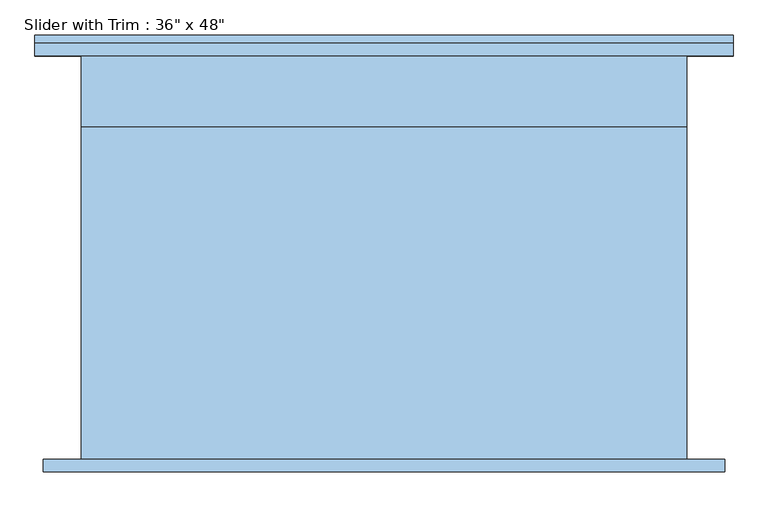
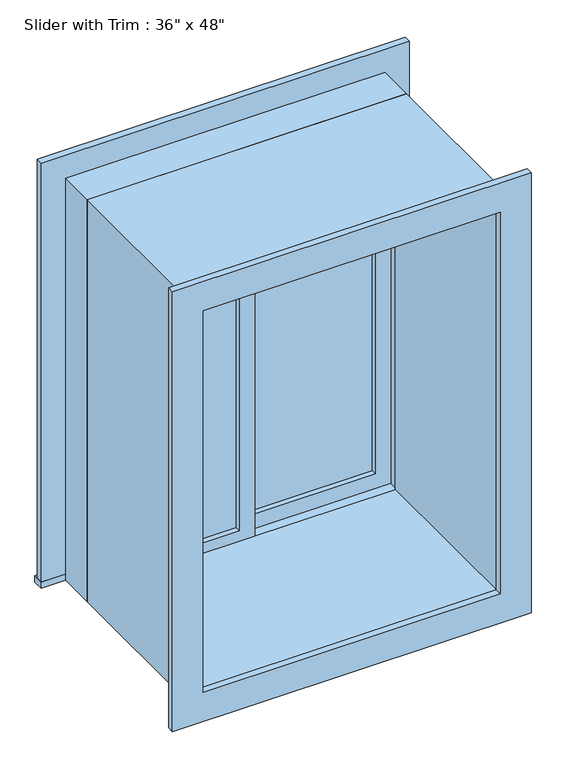
"""IFC4 building model written with IfcOpenShell, lengths in millimetres: window geometry."""

from ifc_helpers import new_model, si_unit, frame, origin, place, context, project, spatial, polyline, outline, extrude, source, transform, mapped, element, save


def window_208eb49b(model_context):
    return source(origin(), model_context, "Body", "SweptSolid", [
        extrude(outline(polyline([(-393.7, 225.425), (-22.225, 225.425), (-22.225, 212.725), (-393.7, 212.725), (-393.7, 225.425)])), frame((0.0, 0.0, 977.9), z_axis=(0.0, 0.0, 1.0), x_axis=(1.0, 0.0, 0.0)), (0.0, 0.0, 1.0), 1092.2),
        extrude(outline(polyline([(2114.55, -438.15), (933.45, -438.15), (933.45, 22.225), (2114.55, 22.225), (2114.55, -438.15)]), holes=[polyline([(2070.1, -393.7), (2070.1, -22.225), (977.9, -22.225), (977.9, -393.7), (2070.1, -393.7)])]), frame((0.0, 196.85, 0.0), z_axis=(0.0, 1.0, 0.0), x_axis=(0.0, 0.0, 1.0)), (0.0, 0.0, 1.0), 44.45),
        extrude(outline(polyline([(-527.05, 336.55), (527.05, 336.55), (527.05, 304.8), (-527.05, 304.8), (-527.05, 336.55)])), frame((0.0, 0.0, 914.4), z_axis=(0.0, 0.0, 1.0), x_axis=(1.0, 0.0, 0.0)), (0.0, 0.0, 1.0), 19.05),
        extrude(outline(polyline([(2114.55, -438.15), (2114.55, 438.15), (933.45, 438.15), (933.45, 527.05), (2203.45, 527.05), (2203.45, -527.05), (933.45, -527.05), (933.45, -438.15), (2114.55, -438.15)])), frame((0.0, 304.8, 0.0), z_axis=(0.0, 1.0, 0.0), x_axis=(0.0, 0.0, 1.0)), (0.0, 0.0, 1.0), 19.05),
        extrude(outline(polyline([(2190.75, 514.35), (2190.75, -514.35), (857.25, -514.35), (857.25, 514.35), (2190.75, 514.35)]), holes=[polyline([(2101.85, 425.45), (946.15, 425.45), (946.15, -425.45), (2101.85, -425.45), (2101.85, 425.45)])]), frame((0.0, -323.85, 0.0), z_axis=(0.0, 1.0, 0.0), x_axis=(0.0, 0.0, 1.0)), (0.0, 0.0, 1.0), 19.05),
        extrude(outline(polyline([(393.7, 257.175), (22.225, 257.175), (22.225, 269.875), (393.7, 269.875), (393.7, 257.175)])), frame((0.0, 0.0, 977.9), z_axis=(0.0, 0.0, 1.0), x_axis=(1.0, 0.0, 0.0)), (0.0, 0.0, 1.0), 1092.2),
        extrude(outline(polyline([(2114.55, -22.225), (933.45, -22.225), (933.45, 438.15), (2114.55, 438.15), (2114.55, -22.225)]), holes=[polyline([(2070.1, 22.225), (2070.1, 393.7), (977.9, 393.7), (977.9, 22.225), (2070.1, 22.225)])]), frame((0.0, 241.3, 0.0), z_axis=(0.0, 1.0, 0.0), x_axis=(0.0, 0.0, 1.0)), (0.0, 0.0, 1.0), 44.45),
        extrude(outline(polyline([(2133.6, -457.2), (914.4, -457.2), (914.4, 457.2), (2133.6, 457.2), (2133.6, -457.2)]), holes=[polyline([(2101.85, -425.45), (2101.85, 425.45), (946.15, 425.45), (946.15, -425.45), (2101.85, -425.45)])]), frame((0.0, -304.8, 0.0), z_axis=(0.0, 1.0, 0.0), x_axis=(0.0, 0.0, 1.0)), (0.0, 0.0, 1.0), 501.65),
        extrude(outline(polyline([(2133.6, 457.2), (2133.6, -457.2), (914.4, -457.2), (914.4, 457.2), (2133.6, 457.2)]), holes=[polyline([(2114.55, 438.15), (933.45, 438.15), (933.45, -438.15), (2114.55, -438.15), (2114.55, 438.15)])]), frame((0.0, 196.85, 0.0), z_axis=(0.0, 1.0, 0.0), x_axis=(0.0, 0.0, 1.0)), (0.0, 0.0, 1.0), 107.95),
    ])


if __name__ == "__main__":
    model = new_model("IFC4")
    model_context = context("Model", 3, world=origin())
    ifc_project = project(units=[si_unit("LENGTHUNIT", "METRE", prefix="MILLI")], contexts=[model_context])
    site = spatial("IfcSite", under=ifc_project)
    building = spatial("IfcBuilding", under=site)
    placement = place(None, origin())
    window_shape = window_208eb49b(model_context)
    element("IfcWindow", 1, ObjectType="Slider with Trim : 36\" x 48\"", at=placement, inside=building, context=model_context, shape_type="MappedRepresentation", body=[
        mapped(window_shape, transform((0.0, 0.0, 0.0), x_axis=(1.0, 0.0, 0.0), y_axis=(0.0, 1.0, 0.0), z_axis=(0.0, 0.0, 1.0))),
    ])
    save(model, "model.ifc")

# Revit data of these elements
# Type "Slider with Trim : 36\" x 48\""
#   Type Mark = "11"
#   Construction Type Id = "GSP4R"
#   Assembly Code = "B2020100"
#   Analytic Construction = "1/8 in Pilkington single glazing"
#   Visual Light Transmittance = 0.9
#   Solar Heat Gain Coefficient = 0.78
#   Heat Transfer Coefficient (U) = 3.6886 W/(m²·K)
#   Height = 4' - 0"
#   Default Sill Height = 3' - 0"
#   Trim Projection - Ext. = 0' - 0 3/4"
#   Trim Projection - Int. = 0' - 0 3/4"
#   Trim Width - Exterior = 0' - 3 1/2"
#   Trim Width - Interior = 0' - 3 1/2"
#   Width = 3' - 0"
#   Window Inset = 0' - 0 3/4"
#   Glass Pane Material = Glass
#   Sash Material = Iron, Ductile
#   Trim Exterior Material = Iron, Ductile
#   Trim Interior Material = Iron, Ductile
#   Wall Closure = (empty or 0)
# Element 1 (IfcWindow, "Slider with Trim : 36\" x 48\"")
#   Materials on its faces: "Iron, Ductile", "Glass"
# Materials
#   "Glass": class "Glass", colour RGB 0 128 192, transparency 0.75, Description = "Soda Lime Glass", Cost = 0
#   "Iron, Ductile": class "Metal", colour RGB 0 0 0, transparency 0, Description = "Ductile cast iron", Cost = 0
